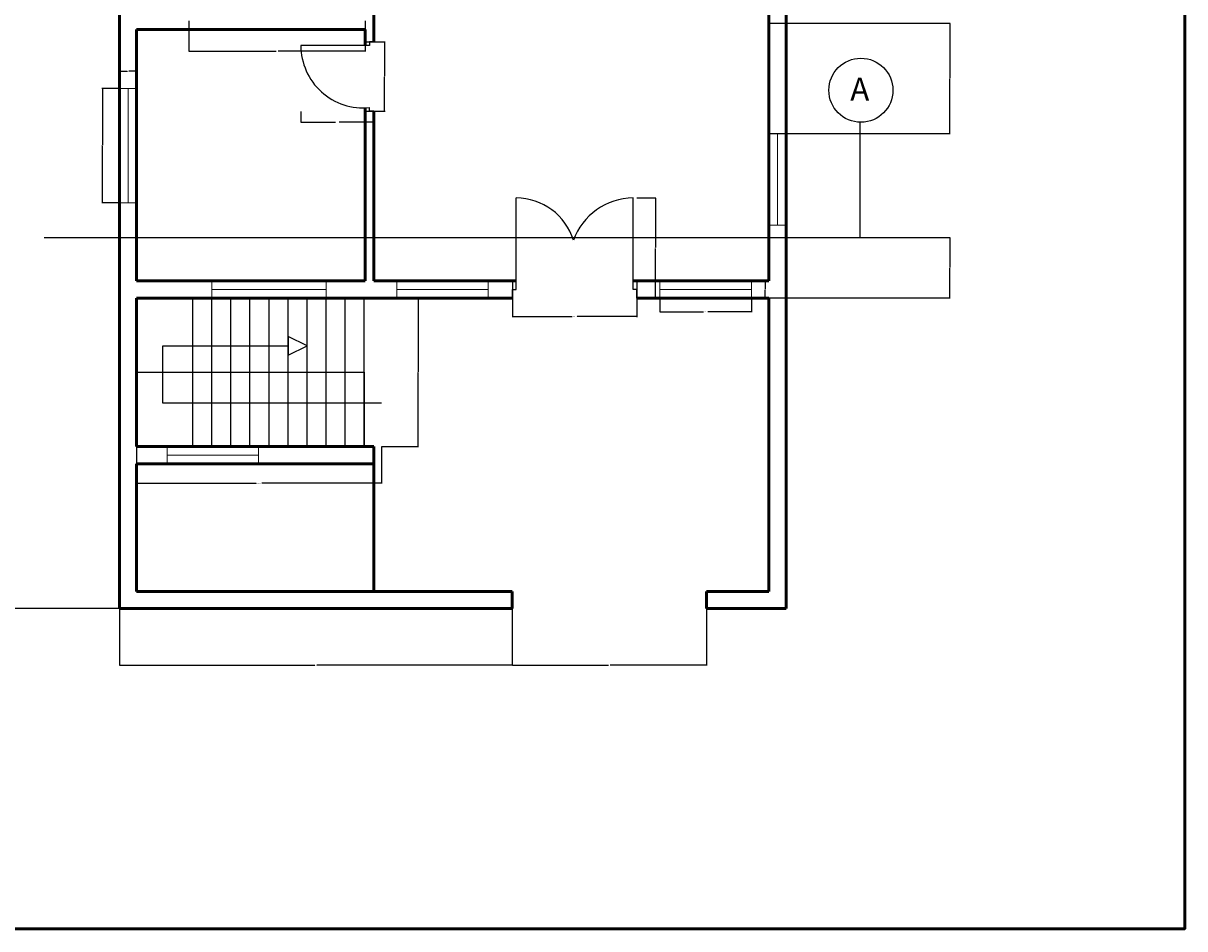
# Model space of a CAD drawing. Units: inches. Extents: x 2268 to 3372, y 1709 to 2892.
# Tile 4 of 6: x 2762 to 3372, y 1709 to 2184. Entities that reach past the tile are written whole.
import ezdxf

# ---------------------------------------------------------------- set-up
doc = ezdxf.new("R2010")
doc.units = ezdxf.units.IN
for name, color, linetype, lineweight in [('A-ANNO-DIMS', 2, 'Continuous', 18), ('A-ANNO-SYMB', 7, 'Continuous', 25), ('A-ANNO-TTLB', 7, 'Continuous', 50), ('A-DOOR', 3, 'Continuous', 25), ('A-FLOR-STRS', 7, 'Continuous', 25), ('A-GLAZ', 4, 'Continuous', 18), ('A-WALL', 7, 'Continuous', 50)]:
    doc.layers.add(name, color=color, linetype=linetype, lineweight=lineweight)
doc.styles.get("Standard").update_dxf_attribs({"font": 'arial.ttf'})
doc.dimstyles.get("Standard").update_dxf_attribs({"dimtxt": 0.18, "dimasz": 0.18, "dimexe": 0.18, "dimexo": 0.0625, "dimgap": 0.09, "dimtad": 0, "dimtih": 1, "dimtoh": 1, "dimdec": 4, "dimzin": 0, "dimdsep": 46, "dimtxsty": 'Standard', "dimcen": 0.09, "dimadec": 0, "dimazin": 0, "dimtfac": 1, "dimtdec": 4, "dimtofl": 0, "dimtmove": 0, "dimatfit": 3, "dimfxl": 1, "dimtolj": 1, "dimtzin": 0, "dimarcsym": 0})

# ---------------------------------------------------------------- blocks, each defined once
blk = doc.blocks.new('DOOR-ENTRY-PAIR')
for p, q in [((2, 4.5), (2, 52.5)), ((63.28, 40.5), (63.28, 52.5)), ((63.28, 4.5), (63.28, 40.5)), ((0, 9), (0, 0)), ((65.28, 9), (65.28, 0)), ((0, 0), (0, 4.5)), ((0, 4.5), (2, 4.5)), ((65.28, 4.5), (63.28, 4.5)), ((65.28, 0), (65.28, 4.5))]:
    blk.add_line(p, q)
for centre, radius, start, end in [((2, 21.15), 31.35, 16.93146, 90), ((63.59, 18.92), 33.58, 90.52016, 160.22729)]:
    blk.add_arc(centre, radius, start, end)
blk = doc.blocks.new('DOOR-BEDROOM-SW')
for p, q in [((36, 34.48), (0, 34.48)), ((33.75, 36.48), (38.25, 36.48)), ((38.25, 36.48), (36, 36.48)), ((36, 36.48), (36, 34.48)), ((33.75, 0), (38.25, 0)), ((36, 0), (36, 2)), ((38.25, 0), (36, 0))]:
    blk.add_line(p, q)
blk.add_arc((32.65, 34.48), 32.65, 180, 275.88229)
blk = doc.blocks.new('WIN-48')
for p, q in [((0, 9), (0, 0)), ((48, 4.5), (48, 9)), ((48, 9), (48, 0)), ((0, 0), (0, 4.5)), ((0, 4.5), (48, 4.5))]:
    blk.add_line(p, q)
blk = doc.blocks.new('WIN-60')
for p, q in [((0, 60), (9, 60)), ((9, 60), (4.5, 60)), ((4.5, 60), (4.5, 0)), ((9, 0), (0, 0)), ((4.5, 0), (9, 0))]:
    blk.add_line(p, q)
blk = doc.blocks.new('STAIR-FRONT-RETURN')
for p, q in [((29.53, 0), (29.53, 78)), ((39.53, 0), (39.53, 78)), ((49.53, 0), (49.53, 78)), ((59.53, 0), (59.53, 78)), ((69.53, 0), (69.53, 78)), ((79.53, 0), (79.53, 78)), ((89.53, 0), (89.53, 78)), ((99.53, 0), (99.53, 78)), ((109.53, 0), (109.53, 78)), ((119.53, 0), (119.53, 78)), ((89.53, 52.91), (79.53, 57.75)), ((79.53, 57.75), (79.53, 48.01)), ((13.79, 22.73), (13.79, 52.91)), ((13.79, 52.91), (79.53, 52.91)), ((79.53, 48.01), (89.53, 52.91)), ((0, 39), (119.53, 39)), ((119.53, 39), (119.53, 0)), ((128.5, 22.73), (13.79, 22.73))]:
    blk.add_line(p, q)
blk = doc.blocks.new('*D26')
at = {"layer": 'A-ANNO-DIMS', "color": 0, "lineweight": -2, "transparency": 16777216}
for p, q in [((3096.79, 2040.11), (3096.79, 2032.8)), ((3144.79, 2040.11), (3144.79, 2032.8)), ((3096.97, 2032.98), (3119.67, 2032.98)), ((3144.61, 2032.98), (3121.91, 2032.98))]:
    blk.add_line(p, q, dxfattribs=at)
at = {"layer": 'A-ANNO-DIMS', "color": 0, "transparency": 16777216}
for points in [[(3096.97, 2033.01), (3096.97, 2032.95), (3096.79, 2032.98)], [(3144.61, 2033.01), (3144.61, 2032.95), (3144.79, 2032.98)]]:
    blk.add_solid(points, dxfattribs=at)
at = {"layer": 'Defpoints', "color": 0, "transparency": 16777216}
for p in [(3096.79, 2040.18), (3144.79, 2040.18), (3144.79, 2032.98)]:
    blk.add_point(p, dxfattribs=at)
at = {"layer": 'A-ANNO-DIMS', "color": 0, "transparency": 16777216, "insert": (3120.79, 2032.98), "char_height": 0.18, "attachment_point": 5}
blk.add_mtext('\\A1;WINDOW 48 TYP.', dxfattribs=at)
blk = doc.blocks.new('*D27')
at = {"layer": 'A-ANNO-DIMS', "color": 0, "lineweight": -2, "transparency": 16777216}
for p, q in [((3144.85, 2049.18), (3152.17, 2049.18)), ((3151.99, 2049), (3151.99, 2044.86)), ((3151.99, 2040.36), (3151.99, 2044.49)), ((3144.85, 2040.18), (3152.17, 2040.18))]:
    blk.add_line(p, q, dxfattribs=at)
at = {"layer": 'A-ANNO-DIMS', "color": 0, "transparency": 16777216}
for points in [[(3151.96, 2049), (3152.02, 2049), (3151.99, 2049.18)], [(3151.96, 2040.36), (3152.02, 2040.36), (3151.99, 2040.18)]]:
    blk.add_solid(points, dxfattribs=at)
at = {"layer": 'Defpoints', "color": 0, "transparency": 16777216}
for p in [(3144.79, 2049.18), (3151.99, 2049.18), (3144.79, 2040.18)]:
    blk.add_point(p, dxfattribs=at)
at = {"layer": 'A-ANNO-DIMS', "color": 0, "transparency": 16777216, "insert": (3151.99, 2044.68), "char_height": 0.18, "attachment_point": 5}
blk.add_mtext('\\A1;9 TYP.', dxfattribs=at)
blk = doc.blocks.new('*D28')
at = {"layer": 'A-ANNO-DIMS', "color": 0, "lineweight": -2, "transparency": 16777216}
for p, q in [((2812.94, 2150.16), (2803.82, 2150.16)), ((2804, 2149.98), (2804, 2120.34)), ((2804, 2090.34), (2804, 2119.98)), ((2812.94, 2090.16), (2803.82, 2090.16))]:
    blk.add_line(p, q, dxfattribs=at)
at = {"layer": 'A-ANNO-DIMS', "color": 0, "transparency": 16777216}
for points in [[(2803.97, 2149.98), (2804.03, 2149.98), (2804, 2150.16)], [(2803.97, 2090.34), (2804.03, 2090.34), (2804, 2090.16)]]:
    blk.add_solid(points, dxfattribs=at)
at = {"layer": 'Defpoints', "color": 0, "transparency": 16777216}
for p in [(2804, 2150.16), (2813, 2150.16), (2813, 2090.16)]:
    blk.add_point(p, dxfattribs=at)
at = {"layer": 'A-ANNO-DIMS', "color": 0, "transparency": 16777216, "insert": (2804, 2120.16), "char_height": 0.18, "attachment_point": 5}
blk.add_mtext('\\A1;WINDOW 60 TYP.', dxfattribs=at)
blk = doc.blocks.new('*D29')
at = {"layer": 'A-ANNO-DIMS', "color": 0, "lineweight": -2, "transparency": 16777216}
for p, q in [((2813, 2150.22), (2813, 2159.34)), ((2813.18, 2159.16), (2817.04, 2159.16)), ((2821.82, 2159.16), (2817.96, 2159.16)), ((2822, 2150.22), (2822, 2159.34))]:
    blk.add_line(p, q, dxfattribs=at)
at = {"layer": 'A-ANNO-DIMS', "color": 0, "transparency": 16777216}
for points in [[(2813.18, 2159.19), (2813.18, 2159.13), (2813, 2159.16)], [(2821.82, 2159.19), (2821.82, 2159.13), (2822, 2159.16)]]:
    blk.add_solid(points, dxfattribs=at)
at = {"layer": 'Defpoints', "color": 0, "transparency": 16777216}
for p in [(2822, 2159.16), (2813, 2150.16), (2822, 2150.16)]:
    blk.add_point(p, dxfattribs=at)
at = {"layer": 'A-ANNO-DIMS', "color": 0, "transparency": 16777216, "insert": (2817.5, 2159.16), "char_height": 0.18, "attachment_point": 5}
blk.add_mtext('\\A1;9 TYP.', dxfattribs=at)
blk = doc.blocks.new('*D30')
at = {"layer": 'A-ANNO-DIMS', "color": 0, "lineweight": -2, "transparency": 16777216}
for p, q in [((3019.35, 2040.11), (3019.35, 2030.2)), ((3084.64, 2040.11), (3084.64, 2030.2)), ((3019.53, 2030.38), (3050.68, 2030.38)), ((3084.46, 2030.38), (3053.31, 2030.38))]:
    blk.add_line(p, q, dxfattribs=at)
at = {"layer": 'A-ANNO-DIMS', "color": 0, "transparency": 16777216}
for points in [[(3019.53, 2030.41), (3019.53, 2030.35), (3019.35, 2030.38)], [(3084.46, 2030.41), (3084.46, 2030.35), (3084.64, 2030.38)]]:
    blk.add_solid(points, dxfattribs=at)
at = {"layer": 'Defpoints', "color": 0, "transparency": 16777216}
for p in [(3019.35, 2040.18), (3084.64, 2040.18), (3084.64, 2030.38)]:
    blk.add_point(p, dxfattribs=at)
at = {"layer": 'A-ANNO-DIMS', "color": 0, "transparency": 16777216, "insert": (3052, 2030.38), "char_height": 0.18, "attachment_point": 5}
blk.add_mtext('\\A1;ENTRY PAIR 65 TYP.', dxfattribs=at)
blk = doc.blocks.new('*D31')
at = {"layer": 'A-ANNO-DIMS', "color": 0, "lineweight": -2, "transparency": 16777216}
for p, q in [((3084.7, 2092.68), (3094.61, 2092.68)), ((3094.43, 2092.5), (3094.43, 2066.61)), ((3094.43, 2040.36), (3094.43, 2066.24)), ((3084.7, 2040.18), (3094.61, 2040.18))]:
    blk.add_line(p, q, dxfattribs=at)
at = {"layer": 'A-ANNO-DIMS', "color": 0, "transparency": 16777216}
for points in [[(3094.4, 2092.5), (3094.46, 2092.5), (3094.43, 2092.68)], [(3094.4, 2040.36), (3094.46, 2040.36), (3094.43, 2040.18)]]:
    blk.add_solid(points, dxfattribs=at)
at = {"layer": 'Defpoints', "color": 0, "transparency": 16777216}
for p in [(3084.64, 2092.68), (3094.43, 2092.68), (3084.64, 2040.18)]:
    blk.add_point(p, dxfattribs=at)
at = {"layer": 'A-ANNO-DIMS', "color": 0, "transparency": 16777216, "insert": (3094.43, 2066.43), "char_height": 0.18, "attachment_point": 5}
blk.add_mtext('\\A1;53 TYP.', dxfattribs=at)
blk = doc.blocks.new('*D40')
at = {"layer": 'A-ANNO-DIMS', "color": 0, "lineweight": -2, "transparency": 16777216}
for p, q in [((2908.25, 2138.11), (2908.25, 2132.25)), ((2946.5, 2138.11), (2946.5, 2132.25)), ((2908.43, 2132.43), (2926.44, 2132.43)), ((2946.32, 2132.43), (2928.31, 2132.43))]:
    blk.add_line(p, q, dxfattribs=at)
at = {"layer": 'A-ANNO-DIMS', "color": 0, "transparency": 16777216}
for points in [[(2908.43, 2132.46), (2908.43, 2132.4), (2908.25, 2132.43)], [(2946.32, 2132.46), (2946.32, 2132.4), (2946.5, 2132.43)]]:
    blk.add_solid(points, dxfattribs=at)
at = {"layer": 'Defpoints', "color": 0, "transparency": 16777216}
for p in [(2908.25, 2138.17), (2946.5, 2138.17), (2946.5, 2132.43)]:
    blk.add_point(p, dxfattribs=at)
at = {"layer": 'A-ANNO-DIMS', "color": 0, "transparency": 16777216, "insert": (2927.38, 2132.43), "char_height": 0.18, "attachment_point": 5}
blk.add_mtext('\\A1;DOOR 38 TYP.', dxfattribs=at)
blk = doc.blocks.new('*D41')
at = {"layer": 'A-ANNO-DIMS', "color": 0, "lineweight": -2, "transparency": 16777216}
for p, q in [((2946.56, 2174.65), (2952.42, 2174.65)), ((2952.24, 2174.47), (2952.24, 2156.59)), ((2952.24, 2138.35), (2952.24, 2156.23)), ((2946.56, 2138.17), (2952.42, 2138.17))]:
    blk.add_line(p, q, dxfattribs=at)
at = {"layer": 'A-ANNO-DIMS', "color": 0, "transparency": 16777216}
for points in [[(2952.21, 2174.47), (2952.27, 2174.47), (2952.24, 2174.65)], [(2952.21, 2138.35), (2952.27, 2138.35), (2952.24, 2138.17)]]:
    blk.add_solid(points, dxfattribs=at)
at = {"layer": 'Defpoints', "color": 0, "transparency": 16777216}
for p in [(2946.5, 2174.65), (2952.24, 2174.65), (2946.5, 2138.17)]:
    blk.add_point(p, dxfattribs=at)
at = {"layer": 'A-ANNO-DIMS', "color": 0, "transparency": 16777216, "insert": (2952.24, 2156.41), "char_height": 0.18, "attachment_point": 5}
blk.add_mtext('\\A1;36 TYP.', dxfattribs=at)
blk = doc.blocks.new('*D56')
at = {"layer": 'A-ANNO-DIMS', "color": 0, "lineweight": -2, "transparency": 16777216}
for p, q in [((2822, 1962.11), (2822, 1942.72)), ((2950.5, 1962.11), (2950.5, 1942.72)), ((2822.18, 1942.9), (2884.69, 1942.9)), ((2950.32, 1942.9), (2887.81, 1942.9))]:
    blk.add_line(p, q, dxfattribs=at)
at = {"layer": 'A-ANNO-DIMS', "color": 0, "transparency": 16777216}
for points in [[(2822.18, 1942.93), (2822.18, 1942.87), (2822, 1942.9)], [(2950.32, 1942.93), (2950.32, 1942.87), (2950.5, 1942.9)]]:
    blk.add_solid(points, dxfattribs=at)
at = {"layer": 'Defpoints', "color": 0, "transparency": 16777216}
for p in [(2822, 1962.18), (2950.5, 1962.18), (2950.5, 1942.9)]:
    blk.add_point(p, dxfattribs=at)
at = {"layer": 'A-ANNO-DIMS', "color": 0, "transparency": 16777216, "insert": (2886.25, 1942.9), "char_height": 0.18, "attachment_point": 5}
blk.add_mtext('\\A1;RETURN STAIR 128 TYP.', dxfattribs=at)
blk = doc.blocks.new('*D57')
at = {"layer": 'A-ANNO-DIMS', "color": 0, "lineweight": -2, "transparency": 16777216}
for p, q in [((2950.56, 2040.18), (2969.96, 2040.18)), ((2969.78, 2040), (2969.78, 2001.36)), ((2969.78, 1962.36), (2969.78, 2000.99)), ((2950.56, 1962.18), (2969.96, 1962.18))]:
    blk.add_line(p, q, dxfattribs=at)
at = {"layer": 'A-ANNO-DIMS', "color": 0, "transparency": 16777216}
for points in [[(2969.75, 2040), (2969.81, 2040), (2969.78, 2040.18)], [(2969.75, 1962.36), (2969.81, 1962.36), (2969.78, 1962.18)]]:
    blk.add_solid(points, dxfattribs=at)
at = {"layer": 'Defpoints', "color": 0, "transparency": 16777216}
for p in [(2950.5, 2040.18), (2969.78, 2040.18), (2950.5, 1962.18)]:
    blk.add_point(p, dxfattribs=at)
at = {"layer": 'A-ANNO-DIMS', "color": 0, "transparency": 16777216, "insert": (2969.78, 2001.18), "char_height": 0.18, "attachment_point": 5}
blk.add_mtext('\\A1;78 TYP.', dxfattribs=at)
blk = doc.blocks.new('*D59')
at = {"layer": 'A-ANNO-DIMS', "color": 0, "lineweight": -2, "transparency": 16777216}
for p, q in [((2849.44, 2185.61), (2849.44, 2169.56)), ((2942, 2185.61), (2942, 2169.56)), ((2849.62, 2169.74), (2895.19, 2169.74)), ((2941.82, 2169.74), (2896.25, 2169.74))]:
    blk.add_line(p, q, dxfattribs=at)
at = {"layer": 'A-ANNO-DIMS', "color": 0, "transparency": 16777216}
for points in [[(2849.62, 2169.77), (2849.62, 2169.71), (2849.44, 2169.74)], [(2941.82, 2169.77), (2941.82, 2169.71), (2942, 2169.74)]]:
    blk.add_solid(points, dxfattribs=at)
at = {"layer": 'Defpoints', "color": 0, "transparency": 16777216}
for p in [(2849.44, 2185.68), (2942, 2185.68), (2942, 2169.74)]:
    blk.add_point(p, dxfattribs=at)
at = {"layer": 'A-ANNO-DIMS', "color": 0, "transparency": 16777216, "insert": (2895.72, 2169.74), "char_height": 0.18, "attachment_point": 5}
blk.add_mtext('\\A1;93 TYP.', dxfattribs=at)
blk = doc.blocks.new('*D90')
at = {"layer": 'A-ANNO-DIMS', "color": 0, "lineweight": -2, "transparency": 16777216}
for p, q in [((2813, 1877.11), (2813, 1847.2)), ((3019.24, 1877.11), (3019.24, 1847.2)), ((2813.18, 1847.38), (2915.66, 1847.38)), ((3019.06, 1847.38), (2916.58, 1847.38))]:
    blk.add_line(p, q, dxfattribs=at)
at = {"layer": 'A-ANNO-DIMS', "color": 0, "transparency": 16777216}
for points in [[(2813.18, 1847.41), (2813.18, 1847.35), (2813, 1847.38)], [(3019.06, 1847.41), (3019.06, 1847.35), (3019.24, 1847.38)]]:
    blk.add_solid(points, dxfattribs=at)
at = {"layer": 'Defpoints', "color": 0, "transparency": 16777216}
for p in [(2813, 1877.18), (3019.24, 1877.18), (3019.24, 1847.38)]:
    blk.add_point(p, dxfattribs=at)
at = {"layer": 'A-ANNO-DIMS', "color": 0, "transparency": 16777216, "insert": (2916.12, 1847.38), "char_height": 0.18, "attachment_point": 5}
blk.add_mtext('\\A1;206.24', dxfattribs=at)
blk = doc.blocks.new('*D91')
at = {"layer": 'A-ANNO-DIMS', "color": 0, "lineweight": -2, "transparency": 16777216}
for p, q in [((3019.24, 1877.11), (3019.24, 1847.2)), ((3121.2, 1877.11), (3121.2, 1847.2)), ((3019.42, 1847.38), (3069.76, 1847.38)), ((3121.02, 1847.38), (3070.67, 1847.38))]:
    blk.add_line(p, q, dxfattribs=at)
at = {"layer": 'A-ANNO-DIMS', "color": 0, "transparency": 16777216}
for points in [[(3019.42, 1847.41), (3019.42, 1847.35), (3019.24, 1847.38)], [(3121.02, 1847.41), (3121.02, 1847.35), (3121.2, 1847.38)]]:
    blk.add_solid(points, dxfattribs=at)
at = {"layer": 'Defpoints', "color": 0, "transparency": 16777216}
for p in [(3019.24, 1877.18), (3121.2, 1877.18), (3121.2, 1847.38)]:
    blk.add_point(p, dxfattribs=at)
at = {"layer": 'A-ANNO-DIMS', "color": 0, "transparency": 16777216, "insert": (3070.22, 1847.38), "char_height": 0.18, "attachment_point": 5}
blk.add_mtext('\\A1;101.96', dxfattribs=at)
blk = doc.blocks.new('*D93')
at = {"layer": 'A-ANNO-DIMS', "color": 0, "lineweight": -2, "transparency": 16777216}
for p, q in [((2812.94, 2463.18), (2743.52, 2463.18)), ((2743.7, 2463), (2743.7, 2170.36)), ((2743.7, 1877.36), (2743.7, 2169.99)), ((2812.94, 1877.18), (2743.52, 1877.18))]:
    blk.add_line(p, q, dxfattribs=at)
at = {"layer": 'A-ANNO-DIMS', "color": 0, "transparency": 16777216}
for points in [[(2743.67, 2463), (2743.73, 2463), (2743.7, 2463.18)], [(2743.67, 1877.36), (2743.73, 1877.36), (2743.7, 1877.18)]]:
    blk.add_solid(points, dxfattribs=at)
at = {"layer": 'Defpoints', "color": 0, "transparency": 16777216}
for p in [(2743.7, 2463.18), (2813, 2463.18), (2813, 1877.18)]:
    blk.add_point(p, dxfattribs=at)
at = {"layer": 'A-ANNO-DIMS', "color": 0, "transparency": 16777216, "insert": (2743.7, 2170.18), "char_height": 0.18, "attachment_point": 5}
blk.add_mtext('\\A1;586', dxfattribs=at)
blk = doc.blocks.new('*D94')
at = {"layer": 'A-ANNO-DIMS', "color": 0, "lineweight": -2, "transparency": 16777216}
for p, q in [((3202.06, 2071.9), (3249.09, 2071.9)), ((3248.91, 2071.72), (3248.91, 2056.22)), ((3248.91, 2040.36), (3248.91, 2055.86)), ((3154.06, 2040.18), (3249.09, 2040.18))]:
    blk.add_line(p, q, dxfattribs=at)
at = {"layer": 'A-ANNO-DIMS', "color": 0, "transparency": 16777216}
for points in [[(3248.88, 2071.72), (3248.94, 2071.72), (3248.91, 2071.9)], [(3248.88, 2040.36), (3248.94, 2040.36), (3248.91, 2040.18)]]:
    blk.add_solid(points, dxfattribs=at)
at = {"layer": 'Defpoints', "color": 0, "transparency": 16777216}
for p in [(3201.99, 2071.9), (3248.91, 2071.9), (3154, 2040.18)]:
    blk.add_point(p, dxfattribs=at)
at = {"layer": 'A-ANNO-DIMS', "color": 0, "transparency": 16777216, "insert": (3248.91, 2056.04), "char_height": 0.18, "attachment_point": 5}
blk.add_mtext('\\A1;31.73', dxfattribs=at)
blk = doc.blocks.new('*D95')
at = {"layer": 'A-ANNO-DIMS', "color": 0, "lineweight": -2, "transparency": 16777216}
for p, q in [((3154.06, 2184.4), (3249.09, 2184.4)), ((3248.91, 2184.22), (3248.91, 2155.61)), ((3248.91, 2126.63), (3248.91, 2155.24)), ((3154.06, 2126.45), (3249.09, 2126.45))]:
    blk.add_line(p, q, dxfattribs=at)
at = {"layer": 'A-ANNO-DIMS', "color": 0, "transparency": 16777216}
for points in [[(3248.88, 2184.22), (3248.94, 2184.22), (3248.91, 2184.4)], [(3248.88, 2126.63), (3248.94, 2126.63), (3248.91, 2126.45)]]:
    blk.add_solid(points, dxfattribs=at)
at = {"layer": 'Defpoints', "color": 0, "transparency": 16777216}
for p in [(3154, 2184.4), (3248.91, 2184.4), (3154, 2126.45)]:
    blk.add_point(p, dxfattribs=at)
at = {"layer": 'A-ANNO-DIMS', "color": 0, "transparency": 16777216, "insert": (3248.91, 2155.43), "char_height": 0.18, "attachment_point": 5}
blk.add_mtext('\\A1;57.96', dxfattribs=at)

msp = doc.modelspace()

# ---------------------------------------------------------------- linework, layer by layer
at = {"layer": 'A-ANNO-SYMB'}
for p, q in [((3201.9948, 2071.9037), (3201.9948, 2132.4003)), ((2773.5041, 2071.9037), (3201.9948, 2071.9037))]:
    msp.add_line(p, q, dxfattribs=at)
msp.add_circle((3202.2872, 2149.2244), 16.8267, dxfattribs=at)
at = {"layer": 'A-ANNO-TTLB'}
msp.add_lwpolyline([(2268.3884, 2892.2471), (3372.3464, 2892.2471), (3372.3464, 1709.0755), (2268.3884, 1709.0755)], close=True, dxfattribs=at)
at = {"layer": 'A-WALL'}
for p, q in [((2813.001, 2463.1756), (2813.001, 1877.1756)), ((3163.001, 2463.1756), (3163.001, 1877.1756)), ((3154.001, 2389.6756), (3154.001, 2049.1756)), ((2946.501, 2192.8278), (2946.501, 2174.6517)), ((2822.001, 2181.1756), (2942.001, 2181.1756)), ((2822.001, 2181.1756), (2822.001, 2049.1756)), ((2942.001, 2181.1756), (2942.001, 2172.6517)), ((2942.001, 2140.0166), (2942.001, 2049.1756)), ((2946.501, 2138.1701), (2946.501, 2049.1756)), ((2822.001, 2049.1756), (2942.001, 2049.1756)), ((2946.501, 2049.1756), (3021.3535, 2049.1756)), ((3082.6386, 2049.1756), (3154.001, 2049.1756)), ((2822.001, 2040.1756), (2942.001, 2040.1756)), ((2822.001, 2040.1756), (2822.001, 1962.1756)), ((2942.001, 2040.1756), (2946.501, 2040.1756)), ((2946.501, 2040.1756), (3019.3535, 2040.1756)), ((3084.6386, 2040.1756), (3154.001, 2040.1756)), ((3154.001, 2040.1756), (3154.001, 1886.1756)), ((2822.001, 1962.1756), (2942.001, 1962.1756)), ((2942.001, 1962.1756), (2942.001, 1962.1756)), ((2942.001, 1962.1756), (2946.501, 1962.1756)), ((2946.501, 1962.1756), (2946.501, 1886.1756)), ((2822.001, 1953.1756), (2942.001, 1953.1756)), ((2822.001, 1953.1756), (2822.001, 1886.1756)), ((2942.001, 1953.1756), (2946.501, 1953.1756)), ((2822.001, 1886.1756), (2942.001, 1886.1756)), ((2942.001, 1886.1756), (2946.501, 1886.1756)), ((3019.2386, 1886.1756), (2946.501, 1886.1756)), ((3019.2386, 1877.1756), (3019.2386, 1886.1756)), ((3121.2007, 1886.1756), (3154.001, 1886.1756)), ((3154.001, 1886.1756), (3121.2007, 1886.1756)), ((3121.2007, 1886.1756), (3121.2007, 1877.1756)), ((2822.001, 1877.1756), (2813.001, 1877.1756)), ((2822.001, 1877.1756), (2942.001, 1877.1756)), ((2946.501, 1877.1756), (2942.001, 1877.1756)), ((2946.501, 1877.1756), (3019.2386, 1877.1756)), ((3121.2007, 1877.1756), (3154.001, 1877.1756)), ((3154.001, 1877.1756), (3163.001, 1877.1756))]:
    msp.add_line(p, q, dxfattribs=at)

# ---------------------------------------------------------------- block references
at = {"layer": 'A-DOOR'}
for name, p in [('DOOR-BEDROOM-SW', (2908.2507, 2138.17)), ('DOOR-ENTRY-PAIR', (3019.3537, 2040.176))]:
    msp.add_blockref(name, p, dxfattribs=at)
at = {"layer": 'A-FLOR-STRS'}
msp.add_blockref('STAIR-FRONT-RETURN', (2822.0007, 1962.176), dxfattribs=at)
at = {"layer": 'A-GLAZ'}
for name, p in [('WIN-60', (2813.0007, 2090.161)), ('WIN-48', (2958.6287, 2040.176)), ('WIN-48', (3096.7917, 2040.176)), ('WIN-48', (2838.0805, 1953.176))]:
    msp.add_blockref(name, p, dxfattribs=at)
for name, p, rotation in [('WIN-48', (3163.0006, 2078.4469), 89.99999999999721), ('WIN-60', (2921.5308, 2040.1753), 89.9999999999986)]:
    msp.add_blockref(name, p, dxfattribs=dict(at, rotation=rotation))

# ---------------------------------------------------------------- texts
at = {"layer": 'A-ANNO-SYMB', "insert": (3196.7327, 2155.8326), "char_height": 12, "attachment_point": 1}
msp.add_mtext_dynamic_manual_height_columns('A', width=16.197641, gutter_width=12.5, heights=[0], dxfattribs=at)

# ---------------------------------------------------------------- dimensions: what is measured, and where the dimension line sits
at = {"layer": 'A-ANNO-DIMS'}
for base, p1, p2, override, picture, middle in [((2743.7041, 2463.1756), (2813.001, 1877.1756), (2813.001, 2463.1756), {"dimdec": 0, "dimlfac": 1, "dimrnd": 0, "dimzin": 0, "dimdsep": 46, "dimlunit": 2}, '*D93', (2743.7041, 2170.1756)), ((3248.9138, 2184.4048), (3154.001, 2126.4464), (3154.001, 2184.4048), {"dimdec": 2, "dimlfac": 1, "dimrnd": 0, "dimzin": 0, "dimdsep": 46, "dimlunit": 2}, '*D95', (3248.9138, 2155.4256)), ((3248.9138, 2071.9037), (3154.001, 2040.1756), (3201.9948, 2071.9037), {"dimdec": 2, "dimlfac": 1, "dimrnd": 0, "dimzin": 0, "dimdsep": 46, "dimlunit": 2}, '*D94', (3248.9138, 2056.0396))]:
    dim = msp.add_linear_dim(base=base, p1=p1, p2=p2, angle=90, dimstyle='Standard', override=override, dxfattribs=at)
    dim.commit()
    dim.dimension.update_dxf_attribs({"geometry": picture, "text_midpoint": middle})
for base, p1, p2, text, picture, middle in [((2942.001, 2169.7422), (2849.4367, 2185.6756), (2942.001, 2185.6756), '<> TYP.', '*D59', (2895.7189, 2169.7422)), ((2822.001, 2159.1612), (2813.001, 2150.1612), (2822.001, 2150.1612), '<> TYP.', '*D29', (2817.501, 2159.1612)), ((2946.501, 2132.4326), (2908.251, 2138.1701), (2946.501, 2138.1701), 'DOOR <> TYP.', '*D40', (2927.376, 2132.4326)), ((3084.6386, 2030.3828), (3019.3535, 2040.1756), (3084.6386, 2040.1756), 'ENTRY PAIR <> TYP.', '*D30', (3051.996, 2030.3828)), ((3144.7912, 2032.9756), (3096.7912, 2040.1756), (3144.7912, 2040.1756), 'WINDOW <> TYP.', '*D26', (3120.7912, 2032.9756)), ((2950.5007, 1942.9006), (2822.001, 1962.1756), (2950.5007, 1962.1756), 'RETURN STAIR <> TYP.', '*D56', (2886.2508, 1942.9006))]:
    dim = msp.add_linear_dim(base=base, p1=p1, p2=p2, text=text, dimstyle='Standard', override={"dimdec": 0, "dimlfac": 1, "dimrnd": 0, "dimzin": 0, "dimdsep": 46, "dimlunit": 2}, dxfattribs=at)
    dim.commit()
    dim.dimension.update_dxf_attribs({"geometry": picture, "text_midpoint": middle})
for base, p1, p2, text, picture, middle in [((2952.2385, 2174.6517), (2946.501, 2138.1701), (2946.501, 2174.6517), '<> TYP.', '*D41', (2952.2385, 2156.4109)), ((2804.001, 2150.1612), (2813.001, 2090.1612), (2813.001, 2150.1612), 'WINDOW <> TYP.', '*D28', (2804.001, 2120.1612)), ((3094.4313408449, 2092.6755932445), (3084.638574026, 2040.1755932445), (3084.638574026, 2092.6755932445), '<> TYP.', '*D31', (3094.4313408449, 2066.4255932445)), ((3151.9912, 2049.1756), (3144.7912, 2040.1756), (3144.7912, 2049.1756), '<> TYP.', '*D27', (3151.9912, 2044.6756)), ((2969.7756, 2040.1756), (2950.5007, 1962.1756), (2950.5007, 2040.1756), '<> TYP.', '*D57', (2969.7756, 2001.1756))]:
    dim = msp.add_linear_dim(base=base, p1=p1, p2=p2, angle=90, text=text, dimstyle='Standard', override={"dimdec": 0, "dimlfac": 1, "dimrnd": 0, "dimzin": 0, "dimdsep": 46, "dimlunit": 2}, dxfattribs=at)
    dim.commit()
    dim.dimension.update_dxf_attribs({"geometry": picture, "text_midpoint": middle})
for base, p1, p2, picture, middle in [((3019.2386, 1847.3756), (2813.001, 1877.1756), (3019.2386, 1877.1756), '*D90', (2916.1198, 1847.3756)), ((3121.2007, 1847.3756), (3019.2386, 1877.1756), (3121.2007, 1877.1756), '*D91', (3070.2196, 1847.3756))]:
    dim = msp.add_linear_dim(base=base, p1=p1, p2=p2, dimstyle='Standard', override={"dimdec": 2, "dimlfac": 1, "dimrnd": 0, "dimzin": 0, "dimdsep": 46, "dimlunit": 2}, dxfattribs=at)
    dim.commit()
    dim.dimension.update_dxf_attribs({"geometry": picture, "text_midpoint": middle})

doc.saveas('drawing.dxf')
